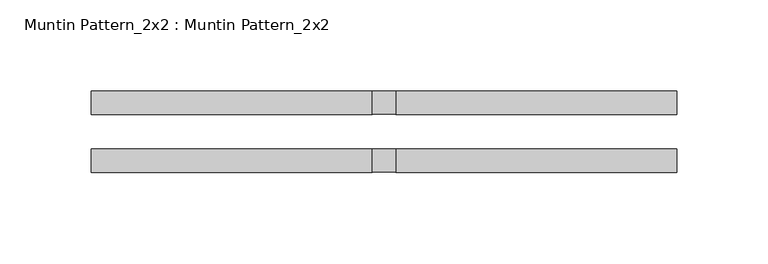
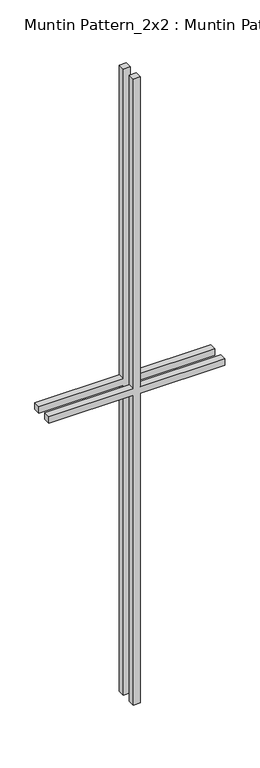
"""IFC4 building model written with IfcOpenShell, lengths in millimetres: proxy geometry, Muntin Pattern_2x2 : Muntin Pattern_2x2."""

from ifc_helpers import new_model, si_unit, frame, origin, place, context, project, spatial, polyline, outline, extrude, source, transform, mapped, element, save


def muntin_pattern_2x2_muntin_pattern_2x2_d319fd2e(model_context):
    return source(origin(), model_context, "Body", "SweptSolid", [
        extrude(outline(polyline([(609.6, -6.35), (609.6, -160.3375), (596.9, -160.3375), (596.9, -6.35), (0.0, -6.35), (0.0, 6.35), (596.9, 6.35), (596.9, 160.3375), (609.6, 160.3375), (609.6, 6.35), (1206.5, 6.35), (1206.5, -6.35), (609.6, -6.35)])), frame((0.0, -22.225, 0.0), z_axis=(0.0, 1.0, 0.0), x_axis=(0.0, 0.0, 1.0)), (0.0, 0.0, 1.0), 12.7),
        extrude(outline(polyline([(609.6, -6.35), (609.6, -160.3375), (596.9, -160.3375), (596.9, -6.35), (0.0, -6.35), (0.0, 6.35), (596.9, 6.35), (596.9, 160.3375), (609.6, 160.3375), (609.6, 6.35), (1206.5, 6.35), (1206.5, -6.35), (609.6, -6.35)])), frame((0.0, 9.525, 0.0), z_axis=(0.0, 1.0, 0.0), x_axis=(0.0, 0.0, 1.0)), (0.0, 0.0, 1.0), 12.7),
    ])


if __name__ == "__main__":
    model = new_model("IFC4")
    model_context = context("Model", 3, world=origin())
    ifc_project = project(units=[si_unit("LENGTHUNIT", "METRE", prefix="MILLI")], contexts=[model_context])
    site = spatial("IfcSite", under=ifc_project)
    building = spatial("IfcBuilding", under=site)
    placement = place(None, origin())
    muntin_pattern_2x2_muntin_pattern_2x2_shape = muntin_pattern_2x2_muntin_pattern_2x2_d319fd2e(model_context)
    element("IfcBuildingElementProxy", 1, Name="Muntin Pattern_2x2 : Muntin Pattern_2x2", ObjectType="Muntin Pattern_2x2 : Muntin Pattern_2x2", at=placement, inside=building, context=model_context, shape_type="MappedRepresentation", body=[
        mapped(muntin_pattern_2x2_muntin_pattern_2x2_shape, transform((0.0, 0.0, 0.0), x_axis=(1.0, 0.0, 0.0), y_axis=(0.0, 1.0, 0.0), z_axis=(0.0, 0.0, 1.0))),
    ])
    save(model, "model.ifc")

# Revit data of these elements
# Type "Muntin Pattern_2x2 : Muntin Pattern_2x2"
#   Width [instance default] = 4' - 0"
#   Thickness = 0' - 0 1/2"
#   Height [instance default] = 4' - 0"
#   Distance = 0' - 0 3/4"
#   Interior Material [instance default] = none
#   Exterior Material [instance default] = none
#   Default Elevation = 0
# Element 1 (IfcBuildingElementProxy, "Muntin Pattern_2x2 : Muntin Pattern_2x2")
#   Width = 1' - 0 5/8"
#   Height = 3' - 11 1/2"
#   Interior Material = Wood - Stained
#   Exterior Material = Clad - White
#   Materials on its faces: "Clad - White", "Wood - Stained"
# Materials
#   "Clad - White": class "Wood", colour RGB 242 242 238, transparency 0, Cost = 0
#   "Wood - Stained": class "Wood", colour RGB 224 178 126, transparency 0, Cost = 0
